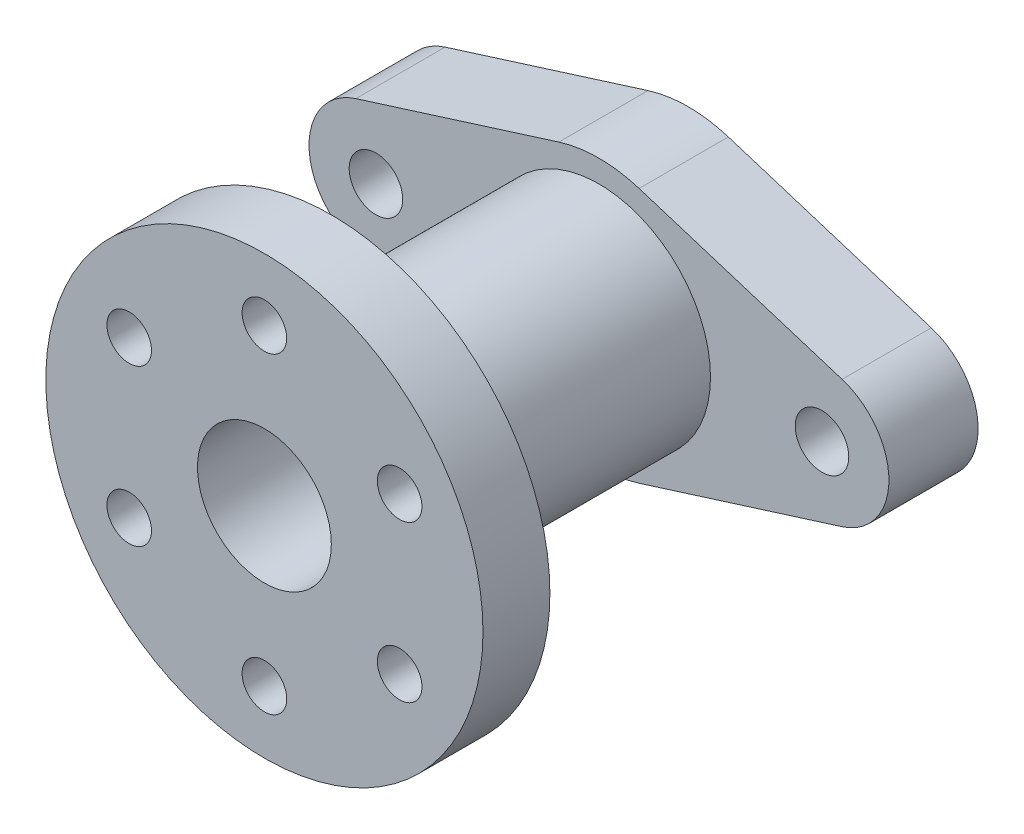
ISO-10303-21;
HEADER;
FILE_DESCRIPTION(('STEP AP214'),'2;1');
FILE_NAME('part.step','',(''),(''),'','','');
FILE_SCHEMA(('AUTOMOTIVE_DESIGN { 1 0 10303 214 1 1 1 1 }'));
ENDSEC;
DATA;
#1=APPLICATION_CONTEXT('core data for automotive mechanical design processes');
#2=APPLICATION_PROTOCOL_DEFINITION('international standard','automotive_design',2000,#1);
#3=PRODUCT_CONTEXT('',#1,'mechanical');
#4=PRODUCT('Part','Part','',(#3));
#5=PRODUCT_RELATED_PRODUCT_CATEGORY('part','',(#4));
#6=PRODUCT_DEFINITION_FORMATION('','',#4);
#7=PRODUCT_DEFINITION_CONTEXT('part definition',#1,'design');
#8=PRODUCT_DEFINITION('design','',#6,#7);
#9=PRODUCT_DEFINITION_SHAPE('','',#8);
#10=(LENGTH_UNIT() NAMED_UNIT(*) SI_UNIT(.MILLI.,.METRE.));
#11=(NAMED_UNIT(*) PLANE_ANGLE_UNIT() SI_UNIT($,.RADIAN.));
#12=(NAMED_UNIT(*) SI_UNIT($,.STERADIAN.) SOLID_ANGLE_UNIT());
#13=UNCERTAINTY_MEASURE_WITH_UNIT(LENGTH_MEASURE(1.E-05),#10,'distance_accuracy_value','');
#14=(GEOMETRIC_REPRESENTATION_CONTEXT(3) GLOBAL_UNCERTAINTY_ASSIGNED_CONTEXT((#13)) GLOBAL_UNIT_ASSIGNED_CONTEXT((#10,
#11,#12)) REPRESENTATION_CONTEXT('',''));
#15=CARTESIAN_POINT('',(0.,0.,0.));
#16=DIRECTION('',(0.,0.,1.));
#17=DIRECTION('',(1.,0.,0.));
#18=AXIS2_PLACEMENT_3D('',#15,#16,#17);
#19=CARTESIAN_POINT('',(0.,0.,20.));
#20=DIRECTION('',(0.,0.,-1.));
#21=DIRECTION('',(-1.,0.,0.));
#22=AXIS2_PLACEMENT_3D('',#19,#20,#21);
#23=CYLINDRICAL_SURFACE('',#22,15.);
#24=CARTESIAN_POINT('',(0.,0.,0.));
#25=DIRECTION('',(0.,0.,1.));
#26=DIRECTION('',(1.,0.,0.));
#27=AXIS2_PLACEMENT_3D('',#24,#25,#26);
#28=CIRCLE('',#27,15.);
#29=CARTESIAN_POINT('',(-4.5,14.3090880212542,0.));
#30=VERTEX_POINT('',#29);
#31=CARTESIAN_POINT('',(-4.5,-14.3090880212542,0.));
#32=VERTEX_POINT('',#31);
#33=EDGE_CURVE('E140',#30,#32,#28,.T.);
#34=ORIENTED_EDGE('',*,*,#33,.T.);
#35=DIRECTION('',(0.,0.,-1.));
#36=VECTOR('',#35,1.);
#37=CARTESIAN_POINT('',(-4.5,-14.3090880212542,20.));
#38=LINE('',#37,#36);
#39=CARTESIAN_POINT('',(-4.5,-14.3090880212542,20.));
#40=VERTEX_POINT('',#39);
#41=EDGE_CURVE('E45',#40,#32,#38,.T.);
#42=ORIENTED_EDGE('',*,*,#41,.F.);
#43=CARTESIAN_POINT('',(0.,0.,20.));
#44=DIRECTION('',(0.,0.,1.));
#45=DIRECTION('',(1.,0.,0.));
#46=AXIS2_PLACEMENT_3D('',#43,#44,#45);
#47=CIRCLE('',#46,15.);
#48=CARTESIAN_POINT('',(-4.5,14.3090880212542,20.));
#49=VERTEX_POINT('',#48);
#50=EDGE_CURVE('E155',#49,#40,#47,.T.);
#51=ORIENTED_EDGE('',*,*,#50,.F.);
#52=DIRECTION('',(0.,0.,-1.));
#53=VECTOR('',#52,1.);
#54=CARTESIAN_POINT('',(-4.5,14.3090880212542,20.));
#55=LINE('',#54,#53);
#56=EDGE_CURVE('E131',#49,#30,#55,.T.);
#57=ORIENTED_EDGE('',*,*,#56,.T.);
#58=EDGE_LOOP('',(#34,#42,#51,#57));
#59=FACE_BOUND('',#58,.T.);
#60=ADVANCED_FACE('F39',(#59),#23,.T.);
#61=CARTESIAN_POINT('',(-4.5,-14.3090880212542,20.));
#62=DIRECTION('',(0.3,0.953939201416946,0.));
#63=DIRECTION('',(-0.953939201416946,0.3,0.));
#64=AXIS2_PLACEMENT_3D('',#61,#62,#63);
#65=PLANE('',#64);
#66=DIRECTION('',(0.953939201416946,-0.3,0.));
#67=VECTOR('',#66,1.);
#68=CARTESIAN_POINT('',(-4.5,-14.3090880212542,0.));
#69=LINE('',#68,#67);
#70=CARTESIAN_POINT('',(41.,-28.6181760425084,0.));
#71=VERTEX_POINT('',#70);
#72=EDGE_CURVE('E138',#32,#71,#69,.T.);
#73=ORIENTED_EDGE('',*,*,#72,.T.);
#74=DIRECTION('',(0.,0.,-1.));
#75=VECTOR('',#74,1.);
#76=CARTESIAN_POINT('',(41.,-28.6181760425084,20.));
#77=LINE('',#76,#75);
#78=CARTESIAN_POINT('',(41.,-28.6181760425084,20.));
#79=VERTEX_POINT('',#78);
#80=EDGE_CURVE('E161',#79,#71,#77,.T.);
#81=ORIENTED_EDGE('',*,*,#80,.F.);
#82=DIRECTION('',(0.953939201416946,-0.3,0.));
#83=VECTOR('',#82,1.);
#84=CARTESIAN_POINT('',(-4.5,-14.3090880212542,20.));
#85=LINE('',#84,#83);
#86=EDGE_CURVE('E99',#40,#79,#85,.T.);
#87=ORIENTED_EDGE('',*,*,#86,.F.);
#88=ORIENTED_EDGE('',*,*,#41,.T.);
#89=EDGE_LOOP('',(#73,#81,#87,#88));
#90=FACE_BOUND('',#89,.T.);
#91=ADVANCED_FACE('F170',(#90),#65,.F.);
#92=CARTESIAN_POINT('',(50.,0.,20.));
#93=DIRECTION('',(0.,0.,-1.));
#94=DIRECTION('',(-1.,0.,0.));
#95=AXIS2_PLACEMENT_3D('',#92,#93,#94);
#96=CYLINDRICAL_SURFACE('',#95,30.);
#97=CARTESIAN_POINT('',(50.,0.,0.));
#98=DIRECTION('',(0.,0.,1.));
#99=DIRECTION('',(1.,0.,0.));
#100=AXIS2_PLACEMENT_3D('',#97,#98,#99);
#101=CIRCLE('',#100,30.);
#102=CARTESIAN_POINT('',(59.,-28.6181760425084,0.));
#103=VERTEX_POINT('',#102);
#104=EDGE_CURVE('E141',#71,#103,#101,.T.);
#105=ORIENTED_EDGE('',*,*,#104,.T.);
#106=DIRECTION('',(0.,0.,-1.));
#107=VECTOR('',#106,1.);
#108=CARTESIAN_POINT('',(59.,-28.6181760425084,20.));
#109=LINE('',#108,#107);
#110=CARTESIAN_POINT('',(59.,-28.6181760425084,20.));
#111=VERTEX_POINT('',#110);
#112=EDGE_CURVE('E157',#111,#103,#109,.T.);
#113=ORIENTED_EDGE('',*,*,#112,.F.);
#114=CARTESIAN_POINT('',(50.,0.,20.));
#115=DIRECTION('',(0.,0.,1.));
#116=DIRECTION('',(1.,0.,0.));
#117=AXIS2_PLACEMENT_3D('',#114,#115,#116);
#118=CIRCLE('',#117,30.);
#119=EDGE_CURVE('E185',#79,#111,#118,.T.);
#120=ORIENTED_EDGE('',*,*,#119,.F.);
#121=ORIENTED_EDGE('',*,*,#80,.T.);
#122=EDGE_LOOP('',(#105,#113,#120,#121));
#123=FACE_BOUND('',#122,.T.);
#124=ADVANCED_FACE('F177',(#123),#96,.T.);
#125=CARTESIAN_POINT('',(59.,-28.6181760425084,20.));
#126=DIRECTION('',(-0.3,0.953939201416946,0.));
#127=DIRECTION('',(-0.953939201416946,-0.3,0.));
#128=AXIS2_PLACEMENT_3D('',#125,#126,#127);
#129=PLANE('',#128);
#130=DIRECTION('',(0.953939201416946,0.3,0.));
#131=VECTOR('',#130,1.);
#132=CARTESIAN_POINT('',(59.,-28.6181760425084,0.));
#133=LINE('',#132,#131);
#134=CARTESIAN_POINT('',(104.5,-14.3090880212542,0.));
#135=VERTEX_POINT('',#134);
#136=EDGE_CURVE('E144',#103,#135,#133,.T.);
#137=ORIENTED_EDGE('',*,*,#136,.T.);
#138=DIRECTION('',(0.,0.,-1.));
#139=VECTOR('',#138,1.);
#140=CARTESIAN_POINT('',(104.5,-14.3090880212542,20.));
#141=LINE('',#140,#139);
#142=CARTESIAN_POINT('',(104.5,-14.3090880212542,20.));
#143=VERTEX_POINT('',#142);
#144=EDGE_CURVE('E156',#143,#135,#141,.T.);
#145=ORIENTED_EDGE('',*,*,#144,.F.);
#146=DIRECTION('',(0.953939201416946,0.3,0.));
#147=VECTOR('',#146,1.);
#148=CARTESIAN_POINT('',(59.,-28.6181760425084,20.));
#149=LINE('',#148,#147);
#150=EDGE_CURVE('E182',#111,#143,#149,.T.);
#151=ORIENTED_EDGE('',*,*,#150,.F.);
#152=ORIENTED_EDGE('',*,*,#112,.T.);
#153=EDGE_LOOP('',(#137,#145,#151,#152));
#154=FACE_BOUND('',#153,.T.);
#155=ADVANCED_FACE('F176',(#154),#129,.F.);
#156=CARTESIAN_POINT('',(100.,0.,20.));
#157=DIRECTION('',(0.,0.,-1.));
#158=DIRECTION('',(-1.,0.,0.));
#159=AXIS2_PLACEMENT_3D('',#156,#157,#158);
#160=CYLINDRICAL_SURFACE('',#159,15.);
#161=CARTESIAN_POINT('',(100.,0.,0.));
#162=DIRECTION('',(0.,0.,1.));
#163=DIRECTION('',(1.,0.,0.));
#164=AXIS2_PLACEMENT_3D('',#161,#162,#163);
#165=CIRCLE('',#164,15.);
#166=CARTESIAN_POINT('',(104.5,14.3090880212542,0.));
#167=VERTEX_POINT('',#166);
#168=EDGE_CURVE('E150',#135,#167,#165,.T.);
#169=ORIENTED_EDGE('',*,*,#168,.T.);
#170=DIRECTION('',(0.,0.,-1.));
#171=VECTOR('',#170,1.);
#172=CARTESIAN_POINT('',(104.5,14.3090880212542,20.));
#173=LINE('',#172,#171);
#174=CARTESIAN_POINT('',(104.5,14.3090880212542,20.));
#175=VERTEX_POINT('',#174);
#176=EDGE_CURVE('E126',#175,#167,#173,.T.);
#177=ORIENTED_EDGE('',*,*,#176,.F.);
#178=CARTESIAN_POINT('',(100.,0.,20.));
#179=DIRECTION('',(0.,0.,1.));
#180=DIRECTION('',(1.,0.,0.));
#181=AXIS2_PLACEMENT_3D('',#178,#179,#180);
#182=CIRCLE('',#181,15.);
#183=EDGE_CURVE('E119',#143,#175,#182,.T.);
#184=ORIENTED_EDGE('',*,*,#183,.F.);
#185=ORIENTED_EDGE('',*,*,#144,.T.);
#186=EDGE_LOOP('',(#169,#177,#184,#185));
#187=FACE_BOUND('',#186,.T.);
#188=ADVANCED_FACE('F293',(#187),#160,.T.);
#189=CARTESIAN_POINT('',(59.,28.6181760425084,20.));
#190=DIRECTION('',(-0.3,-0.953939201416946,0.));
#191=DIRECTION('',(0.953939201416946,-0.3,0.));
#192=AXIS2_PLACEMENT_3D('',#189,#190,#191);
#193=PLANE('',#192);
#194=DIRECTION('',(-0.953939201416946,0.3,0.));
#195=VECTOR('',#194,1.);
#196=CARTESIAN_POINT('',(59.,28.6181760425084,0.));
#197=LINE('',#196,#195);
#198=CARTESIAN_POINT('',(59.,28.6181760425084,0.));
#199=VERTEX_POINT('',#198);
#200=EDGE_CURVE('E130',#167,#199,#197,.T.);
#201=ORIENTED_EDGE('',*,*,#200,.T.);
#202=DIRECTION('',(0.,0.,-1.));
#203=VECTOR('',#202,1.);
#204=CARTESIAN_POINT('',(59.,28.6181760425084,20.));
#205=LINE('',#204,#203);
#206=CARTESIAN_POINT('',(59.,28.6181760425084,20.));
#207=VERTEX_POINT('',#206);
#208=EDGE_CURVE('E121',#207,#199,#205,.T.);
#209=ORIENTED_EDGE('',*,*,#208,.F.);
#210=DIRECTION('',(-0.953939201416946,0.3,0.));
#211=VECTOR('',#210,1.);
#212=CARTESIAN_POINT('',(59.,28.6181760425084,20.));
#213=LINE('',#212,#211);
#214=EDGE_CURVE('E114',#175,#207,#213,.T.);
#215=ORIENTED_EDGE('',*,*,#214,.F.);
#216=ORIENTED_EDGE('',*,*,#176,.T.);
#217=EDGE_LOOP('',(#201,#209,#215,#216));
#218=FACE_BOUND('',#217,.T.);
#219=ADVANCED_FACE('F123',(#218),#193,.F.);
#220=CARTESIAN_POINT('',(50.,0.,20.));
#221=DIRECTION('',(0.,0.,-1.));
#222=DIRECTION('',(-1.,0.,0.));
#223=AXIS2_PLACEMENT_3D('',#220,#221,#222);
#224=CYLINDRICAL_SURFACE('',#223,30.);
#225=CARTESIAN_POINT('',(50.,0.,0.));
#226=DIRECTION('',(0.,0.,1.));
#227=DIRECTION('',(1.,0.,0.));
#228=AXIS2_PLACEMENT_3D('',#225,#226,#227);
#229=CIRCLE('',#228,30.);
#230=CARTESIAN_POINT('',(41.,28.6181760425084,0.));
#231=VERTEX_POINT('',#230);
#232=EDGE_CURVE('E83',#199,#231,#229,.T.);
#233=ORIENTED_EDGE('',*,*,#232,.T.);
#234=DIRECTION('',(0.,0.,-1.));
#235=VECTOR('',#234,1.);
#236=CARTESIAN_POINT('',(41.,28.6181760425084,20.));
#237=LINE('',#236,#235);
#238=CARTESIAN_POINT('',(41.,28.6181760425084,20.));
#239=VERTEX_POINT('',#238);
#240=EDGE_CURVE('E129',#239,#231,#237,.T.);
#241=ORIENTED_EDGE('',*,*,#240,.F.);
#242=CARTESIAN_POINT('',(50.,0.,20.));
#243=DIRECTION('',(0.,0.,1.));
#244=DIRECTION('',(1.,0.,0.));
#245=AXIS2_PLACEMENT_3D('',#242,#243,#244);
#246=CIRCLE('',#245,30.);
#247=EDGE_CURVE('E120',#207,#239,#246,.T.);
#248=ORIENTED_EDGE('',*,*,#247,.F.);
#249=ORIENTED_EDGE('',*,*,#208,.T.);
#250=EDGE_LOOP('',(#233,#241,#248,#249));
#251=FACE_BOUND('',#250,.T.);
#252=ADVANCED_FACE('F133',(#251),#224,.T.);
#253=CARTESIAN_POINT('',(-4.5,14.3090880212542,20.));
#254=DIRECTION('',(0.3,-0.953939201416946,0.));
#255=DIRECTION('',(0.953939201416946,0.3,0.));
#256=AXIS2_PLACEMENT_3D('',#253,#254,#255);
#257=PLANE('',#256);
#258=DIRECTION('',(-0.953939201416946,-0.3,0.));
#259=VECTOR('',#258,1.);
#260=CARTESIAN_POINT('',(-4.5,14.3090880212542,0.));
#261=LINE('',#260,#259);
#262=EDGE_CURVE('E93',#231,#30,#261,.T.);
#263=ORIENTED_EDGE('',*,*,#262,.T.);
#264=ORIENTED_EDGE('',*,*,#56,.F.);
#265=DIRECTION('',(-0.953939201416946,-0.3,0.));
#266=VECTOR('',#265,1.);
#267=CARTESIAN_POINT('',(-4.5,14.3090880212542,20.));
#268=LINE('',#267,#266);
#269=EDGE_CURVE('E57',#239,#49,#268,.T.);
#270=ORIENTED_EDGE('',*,*,#269,.F.);
#271=ORIENTED_EDGE('',*,*,#240,.T.);
#272=EDGE_LOOP('',(#263,#264,#270,#271));
#273=FACE_BOUND('',#272,.T.);
#274=ADVANCED_FACE('F265',(#273),#257,.F.);
#275=CARTESIAN_POINT('',(0.,0.,20.));
#276=DIRECTION('',(0.,0.,1.));
#277=DIRECTION('',(1.,0.,0.));
#278=AXIS2_PLACEMENT_3D('',#275,#276,#277);
#279=PLANE('',#278);
#280=CARTESIAN_POINT('',(0.,0.,20.));
#281=DIRECTION('',(0.,0.,1.));
#282=DIRECTION('',(1.,0.,0.));
#283=AXIS2_PLACEMENT_3D('',#280,#281,#282);
#284=CIRCLE('',#283,6.);
#285=CARTESIAN_POINT('',(6.,0.,20.));
#286=VERTEX_POINT('',#285);
#287=EDGE_CURVE('E242',#286,#286,#284,.T.);
#288=ORIENTED_EDGE('',*,*,#287,.F.);
#289=EDGE_LOOP('',(#288));
#290=FACE_BOUND('',#289,.T.);
#291=CARTESIAN_POINT('',(100.,0.,20.));
#292=DIRECTION('',(0.,0.,1.));
#293=DIRECTION('',(1.,0.,0.));
#294=AXIS2_PLACEMENT_3D('',#291,#292,#293);
#295=CIRCLE('',#294,6.);
#296=CARTESIAN_POINT('',(106.,0.,20.));
#297=VERTEX_POINT('',#296);
#298=EDGE_CURVE('E239',#297,#297,#295,.T.);
#299=ORIENTED_EDGE('',*,*,#298,.F.);
#300=EDGE_LOOP('',(#299));
#301=FACE_BOUND('',#300,.T.);
#302=CARTESIAN_POINT('',(50.,0.,20.));
#303=DIRECTION('',(0.,0.,1.));
#304=DIRECTION('',(1.,0.,0.));
#305=AXIS2_PLACEMENT_3D('',#302,#303,#304);
#306=CIRCLE('',#305,25.);
#307=CARTESIAN_POINT('',(75.,0.,20.));
#308=VERTEX_POINT('',#307);
#309=EDGE_CURVE('E11',#308,#308,#306,.T.);
#310=ORIENTED_EDGE('',*,*,#309,.F.);
#311=EDGE_LOOP('',(#310));
#312=FACE_BOUND('',#311,.T.);
#313=ORIENTED_EDGE('',*,*,#50,.T.);
#314=ORIENTED_EDGE('',*,*,#86,.T.);
#315=ORIENTED_EDGE('',*,*,#119,.T.);
#316=ORIENTED_EDGE('',*,*,#150,.T.);
#317=ORIENTED_EDGE('',*,*,#183,.T.);
#318=ORIENTED_EDGE('',*,*,#214,.T.);
#319=ORIENTED_EDGE('',*,*,#247,.T.);
#320=ORIENTED_EDGE('',*,*,#269,.T.);
#321=EDGE_LOOP('',(#313,#314,#315,#316,#317,#318,#319,#320));
#322=FACE_BOUND('',#321,.T.);
#323=ADVANCED_FACE('F113',(#290,#301,#312,#322),#279,.T.);
#324=CARTESIAN_POINT('',(0.,0.,0.));
#325=DIRECTION('',(0.,0.,1.));
#326=DIRECTION('',(1.,0.,0.));
#327=AXIS2_PLACEMENT_3D('',#324,#325,#326);
#328=PLANE('',#327);
#329=CARTESIAN_POINT('',(50.,0.,0.));
#330=DIRECTION('',(0.,0.,1.));
#331=DIRECTION('',(1.,0.,0.));
#332=AXIS2_PLACEMENT_3D('',#329,#330,#331);
#333=CIRCLE('',#332,15.);
#334=CARTESIAN_POINT('',(65.,0.,0.));
#335=VERTEX_POINT('',#334);
#336=EDGE_CURVE('E199',#335,#335,#333,.T.);
#337=ORIENTED_EDGE('',*,*,#336,.T.);
#338=EDGE_LOOP('',(#337));
#339=FACE_BOUND('',#338,.T.);
#340=ORIENTED_EDGE('',*,*,#33,.F.);
#341=ORIENTED_EDGE('',*,*,#262,.F.);
#342=ORIENTED_EDGE('',*,*,#232,.F.);
#343=ORIENTED_EDGE('',*,*,#200,.F.);
#344=ORIENTED_EDGE('',*,*,#168,.F.);
#345=ORIENTED_EDGE('',*,*,#136,.F.);
#346=ORIENTED_EDGE('',*,*,#104,.F.);
#347=ORIENTED_EDGE('',*,*,#72,.F.);
#348=EDGE_LOOP('',(#340,#341,#342,#343,#344,#345,#346,#347));
#349=FACE_BOUND('',#348,.T.);
#350=ADVANCED_FACE('F175',(#339,#349),#328,.F.);
#351=CARTESIAN_POINT('',(50.,0.,80.));
#352=DIRECTION('',(0.,0.,-1.));
#353=DIRECTION('',(-1.,0.,0.));
#354=AXIS2_PLACEMENT_3D('',#351,#352,#353);
#355=CYLINDRICAL_SURFACE('',#354,25.);
#356=CARTESIAN_POINT('',(50.,0.,80.));
#357=DIRECTION('',(0.,0.,1.));
#358=DIRECTION('',(1.,0.,0.));
#359=AXIS2_PLACEMENT_3D('',#356,#357,#358);
#360=CIRCLE('',#359,25.);
#361=CARTESIAN_POINT('',(75.,0.,80.));
#362=VERTEX_POINT('',#361);
#363=EDGE_CURVE('E143',#362,#362,#360,.T.);
#364=ORIENTED_EDGE('',*,*,#363,.F.);
#365=EDGE_LOOP('',(#364));
#366=FACE_BOUND('',#365,.T.);
#367=ORIENTED_EDGE('',*,*,#309,.T.);
#368=EDGE_LOOP('',(#367));
#369=FACE_BOUND('',#368,.T.);
#370=ADVANCED_FACE('F268',(#366,#369),#355,.T.);
#371=CARTESIAN_POINT('',(50.,0.,95.));
#372=DIRECTION('',(0.,0.,-1.));
#373=DIRECTION('',(-1.,0.,0.));
#374=AXIS2_PLACEMENT_3D('',#371,#372,#373);
#375=CYLINDRICAL_SURFACE('',#374,49.);
#376=CARTESIAN_POINT('',(50.,0.,95.));
#377=DIRECTION('',(0.,0.,1.));
#378=DIRECTION('',(1.,0.,0.));
#379=AXIS2_PLACEMENT_3D('',#376,#377,#378);
#380=CIRCLE('',#379,49.);
#381=CARTESIAN_POINT('',(99.,0.,95.));
#382=VERTEX_POINT('',#381);
#383=EDGE_CURVE('E187',#382,#382,#380,.T.);
#384=ORIENTED_EDGE('',*,*,#383,.F.);
#385=EDGE_LOOP('',(#384));
#386=FACE_BOUND('',#385,.T.);
#387=CARTESIAN_POINT('',(50.,0.,80.));
#388=DIRECTION('',(0.,0.,1.));
#389=DIRECTION('',(1.,0.,0.));
#390=AXIS2_PLACEMENT_3D('',#387,#388,#389);
#391=CIRCLE('',#390,49.);
#392=CARTESIAN_POINT('',(99.,0.,80.));
#393=VERTEX_POINT('',#392);
#394=EDGE_CURVE('E192',#393,#393,#391,.T.);
#395=ORIENTED_EDGE('',*,*,#394,.T.);
#396=EDGE_LOOP('',(#395));
#397=FACE_BOUND('',#396,.T.);
#398=ADVANCED_FACE('F269',(#386,#397),#375,.T.);
#399=CARTESIAN_POINT('',(50.,0.,95.));
#400=DIRECTION('',(0.,0.,1.));
#401=DIRECTION('',(1.,0.,0.));
#402=AXIS2_PLACEMENT_3D('',#399,#400,#401);
#403=PLANE('',#402);
#404=CARTESIAN_POINT('',(19.6891108675449,17.5000000000003,95.));
#405=DIRECTION('',(0.,0.,1.));
#406=DIRECTION('',(0.50000000000001,0.866025403784433,0.));
#407=AXIS2_PLACEMENT_3D('',#404,#405,#406);
#408=CIRCLE('',#407,5.00000000000001);
#409=CARTESIAN_POINT('',(22.1891108675449,21.8301270189225,95.));
#410=VERTEX_POINT('',#409);
#411=EDGE_CURVE('E214',#410,#410,#408,.T.);
#412=ORIENTED_EDGE('',*,*,#411,.F.);
#413=EDGE_LOOP('',(#412));
#414=FACE_BOUND('',#413,.T.);
#415=CARTESIAN_POINT('',(19.6891108675445,-17.4999999999997,95.));
#416=DIRECTION('',(0.,0.,1.));
#417=DIRECTION('',(-0.499999999999992,0.866025403784443,0.));
#418=AXIS2_PLACEMENT_3D('',#415,#416,#417);
#419=CIRCLE('',#418,5.00000000000001);
#420=CARTESIAN_POINT('',(17.1891108675445,-13.1698729810775,95.));
#421=VERTEX_POINT('',#420);
#422=EDGE_CURVE('E225',#421,#421,#419,.T.);
#423=ORIENTED_EDGE('',*,*,#422,.F.);
#424=EDGE_LOOP('',(#423));
#425=FACE_BOUND('',#424,.T.);
#426=CARTESIAN_POINT('',(50.,-35.,95.));
#427=DIRECTION('',(0.,0.,1.));
#428=DIRECTION('',(-1.,0.,0.));
#429=AXIS2_PLACEMENT_3D('',#426,#427,#428);
#430=CIRCLE('',#429,5.00000000000001);
#431=CARTESIAN_POINT('',(45.,-35.,95.));
#432=VERTEX_POINT('',#431);
#433=EDGE_CURVE('E226',#432,#432,#430,.T.);
#434=ORIENTED_EDGE('',*,*,#433,.F.);
#435=EDGE_LOOP('',(#434));
#436=FACE_BOUND('',#435,.T.);
#437=CARTESIAN_POINT('',(80.3108891324553,-17.5000000000001,95.));
#438=DIRECTION('',(0.,0.,1.));
#439=DIRECTION('',(-0.500000000000004,-0.866025403784436,0.));
#440=AXIS2_PLACEMENT_3D('',#437,#438,#439);
#441=CIRCLE('',#440,5.00000000000001);
#442=CARTESIAN_POINT('',(77.8108891324552,-21.8301270189223,95.));
#443=VERTEX_POINT('',#442);
#444=EDGE_CURVE('E231',#443,#443,#441,.T.);
#445=ORIENTED_EDGE('',*,*,#444,.F.);
#446=EDGE_LOOP('',(#445));
#447=FACE_BOUND('',#446,.T.);
#448=CARTESIAN_POINT('',(80.3108891324554,17.4999999999999,95.));
#449=DIRECTION('',(0.,0.,1.));
#450=DIRECTION('',(0.499999999999998,-0.86602540378444,0.));
#451=AXIS2_PLACEMENT_3D('',#448,#449,#450);
#452=CIRCLE('',#451,5.00000000000001);
#453=CARTESIAN_POINT('',(82.8108891324554,13.1698729810777,95.));
#454=VERTEX_POINT('',#453);
#455=EDGE_CURVE('E207',#454,#454,#452,.T.);
#456=ORIENTED_EDGE('',*,*,#455,.F.);
#457=EDGE_LOOP('',(#456));
#458=FACE_BOUND('',#457,.T.);
#459=CARTESIAN_POINT('',(50.,0.,95.));
#460=DIRECTION('',(0.,0.,1.));
#461=DIRECTION('',(1.,0.,0.));
#462=AXIS2_PLACEMENT_3D('',#459,#460,#461);
#463=CIRCLE('',#462,15.);
#464=CARTESIAN_POINT('',(65.,0.,95.));
#465=VERTEX_POINT('',#464);
#466=EDGE_CURVE('E201',#465,#465,#463,.T.);
#467=ORIENTED_EDGE('',*,*,#466,.F.);
#468=EDGE_LOOP('',(#467));
#469=FACE_BOUND('',#468,.T.);
#470=CARTESIAN_POINT('',(50.,35.,95.));
#471=DIRECTION('',(0.,0.,1.));
#472=DIRECTION('',(1.,0.,0.));
#473=AXIS2_PLACEMENT_3D('',#470,#471,#472);
#474=CIRCLE('',#473,5.00000000000001);
#475=CARTESIAN_POINT('',(55.,35.,95.));
#476=VERTEX_POINT('',#475);
#477=EDGE_CURVE('E197',#476,#476,#474,.T.);
#478=ORIENTED_EDGE('',*,*,#477,.F.);
#479=EDGE_LOOP('',(#478));
#480=FACE_BOUND('',#479,.T.);
#481=ORIENTED_EDGE('',*,*,#383,.T.);
#482=EDGE_LOOP('',(#481));
#483=FACE_BOUND('',#482,.T.);
#484=ADVANCED_FACE('F280',(#414,#425,#436,#447,#458,#469,#480,#483),#403,.T.);
#485=CARTESIAN_POINT('',(50.,0.,80.));
#486=DIRECTION('',(0.,0.,1.));
#487=DIRECTION('',(1.,0.,0.));
#488=AXIS2_PLACEMENT_3D('',#485,#486,#487);
#489=PLANE('',#488);
#490=CARTESIAN_POINT('',(19.6891108675449,17.5000000000003,80.));
#491=DIRECTION('',(0.,0.,1.));
#492=DIRECTION('',(0.50000000000001,0.866025403784433,0.));
#493=AXIS2_PLACEMENT_3D('',#490,#491,#492);
#494=CIRCLE('',#493,5.00000000000001);
#495=CARTESIAN_POINT('',(22.1891108675449,21.8301270189225,80.));
#496=VERTEX_POINT('',#495);
#497=EDGE_CURVE('E217',#496,#496,#494,.T.);
#498=ORIENTED_EDGE('',*,*,#497,.T.);
#499=EDGE_LOOP('',(#498));
#500=FACE_BOUND('',#499,.T.);
#501=CARTESIAN_POINT('',(19.6891108675445,-17.4999999999997,80.));
#502=DIRECTION('',(0.,0.,1.));
#503=DIRECTION('',(-0.499999999999992,0.866025403784443,0.));
#504=AXIS2_PLACEMENT_3D('',#501,#502,#503);
#505=CIRCLE('',#504,5.00000000000001);
#506=CARTESIAN_POINT('',(17.1891108675445,-13.1698729810775,80.));
#507=VERTEX_POINT('',#506);
#508=EDGE_CURVE('E223',#507,#507,#505,.T.);
#509=ORIENTED_EDGE('',*,*,#508,.T.);
#510=EDGE_LOOP('',(#509));
#511=FACE_BOUND('',#510,.T.);
#512=CARTESIAN_POINT('',(50.,-35.,80.));
#513=DIRECTION('',(0.,0.,1.));
#514=DIRECTION('',(-1.,0.,0.));
#515=AXIS2_PLACEMENT_3D('',#512,#513,#514);
#516=CIRCLE('',#515,5.00000000000001);
#517=CARTESIAN_POINT('',(45.,-35.,80.));
#518=VERTEX_POINT('',#517);
#519=EDGE_CURVE('E232',#518,#518,#516,.T.);
#520=ORIENTED_EDGE('',*,*,#519,.T.);
#521=EDGE_LOOP('',(#520));
#522=FACE_BOUND('',#521,.T.);
#523=CARTESIAN_POINT('',(80.3108891324553,-17.5000000000001,80.));
#524=DIRECTION('',(0.,0.,1.));
#525=DIRECTION('',(-0.500000000000004,-0.866025403784436,0.));
#526=AXIS2_PLACEMENT_3D('',#523,#524,#525);
#527=CIRCLE('',#526,5.00000000000001);
#528=CARTESIAN_POINT('',(77.8108891324552,-21.8301270189223,80.));
#529=VERTEX_POINT('',#528);
#530=EDGE_CURVE('E215',#529,#529,#527,.T.);
#531=ORIENTED_EDGE('',*,*,#530,.T.);
#532=EDGE_LOOP('',(#531));
#533=FACE_BOUND('',#532,.T.);
#534=CARTESIAN_POINT('',(80.3108891324554,17.4999999999999,80.));
#535=DIRECTION('',(0.,0.,1.));
#536=DIRECTION('',(0.499999999999998,-0.86602540378444,0.));
#537=AXIS2_PLACEMENT_3D('',#534,#535,#536);
#538=CIRCLE('',#537,5.00000000000001);
#539=CARTESIAN_POINT('',(82.8108891324554,13.1698729810777,80.));
#540=VERTEX_POINT('',#539);
#541=EDGE_CURVE('E206',#540,#540,#538,.T.);
#542=ORIENTED_EDGE('',*,*,#541,.T.);
#543=EDGE_LOOP('',(#542));
#544=FACE_BOUND('',#543,.T.);
#545=CARTESIAN_POINT('',(50.,35.,80.));
#546=DIRECTION('',(0.,0.,1.));
#547=DIRECTION('',(1.,0.,0.));
#548=AXIS2_PLACEMENT_3D('',#545,#546,#547);
#549=CIRCLE('',#548,5.00000000000001);
#550=CARTESIAN_POINT('',(55.,35.,80.));
#551=VERTEX_POINT('',#550);
#552=EDGE_CURVE('E191',#551,#551,#549,.T.);
#553=ORIENTED_EDGE('',*,*,#552,.T.);
#554=EDGE_LOOP('',(#553));
#555=FACE_BOUND('',#554,.T.);
#556=ORIENTED_EDGE('',*,*,#363,.T.);
#557=EDGE_LOOP('',(#556));
#558=FACE_BOUND('',#557,.T.);
#559=ORIENTED_EDGE('',*,*,#394,.F.);
#560=EDGE_LOOP('',(#559));
#561=FACE_BOUND('',#560,.T.);
#562=ADVANCED_FACE('F371',(#500,#511,#522,#533,#544,#555,#558,#561),#489,.F.);
#563=CARTESIAN_POINT('',(50.,35.,80.));
#564=DIRECTION('',(0.,0.,1.));
#565=DIRECTION('',(1.,0.,0.));
#566=AXIS2_PLACEMENT_3D('',#563,#564,#565);
#567=CYLINDRICAL_SURFACE('',#566,5.00000000000001);
#568=ORIENTED_EDGE('',*,*,#552,.F.);
#569=EDGE_LOOP('',(#568));
#570=FACE_BOUND('',#569,.T.);
#571=ORIENTED_EDGE('',*,*,#477,.T.);
#572=EDGE_LOOP('',(#571));
#573=FACE_BOUND('',#572,.T.);
#574=ADVANCED_FACE('F379',(#570,#573),#567,.F.);
#575=CARTESIAN_POINT('',(50.,0.,0.));
#576=DIRECTION('',(0.,0.,1.));
#577=DIRECTION('',(1.,0.,0.));
#578=AXIS2_PLACEMENT_3D('',#575,#576,#577);
#579=CYLINDRICAL_SURFACE('',#578,15.);
#580=ORIENTED_EDGE('',*,*,#336,.F.);
#581=EDGE_LOOP('',(#580));
#582=FACE_BOUND('',#581,.T.);
#583=ORIENTED_EDGE('',*,*,#466,.T.);
#584=EDGE_LOOP('',(#583));
#585=FACE_BOUND('',#584,.T.);
#586=ADVANCED_FACE('F386',(#582,#585),#579,.F.);
#587=CARTESIAN_POINT('',(80.3108891324554,17.4999999999999,80.));
#588=DIRECTION('',(0.,0.,1.));
#589=DIRECTION('',(1.,0.,0.));
#590=AXIS2_PLACEMENT_3D('',#587,#588,#589);
#591=CYLINDRICAL_SURFACE('',#590,5.00000000000001);
#592=ORIENTED_EDGE('',*,*,#541,.F.);
#593=EDGE_LOOP('',(#592));
#594=FACE_BOUND('',#593,.T.);
#595=ORIENTED_EDGE('',*,*,#455,.T.);
#596=EDGE_LOOP('',(#595));
#597=FACE_BOUND('',#596,.T.);
#598=ADVANCED_FACE('F399',(#594,#597),#591,.F.);
#599=CARTESIAN_POINT('',(80.3108891324553,-17.5000000000001,80.));
#600=DIRECTION('',(0.,0.,1.));
#601=DIRECTION('',(1.,0.,0.));
#602=AXIS2_PLACEMENT_3D('',#599,#600,#601);
#603=CYLINDRICAL_SURFACE('',#602,5.00000000000001);
#604=ORIENTED_EDGE('',*,*,#530,.F.);
#605=EDGE_LOOP('',(#604));
#606=FACE_BOUND('',#605,.T.);
#607=ORIENTED_EDGE('',*,*,#444,.T.);
#608=EDGE_LOOP('',(#607));
#609=FACE_BOUND('',#608,.T.);
#610=ADVANCED_FACE('F410',(#606,#609),#603,.F.);
#611=CARTESIAN_POINT('',(50.,-35.,80.));
#612=DIRECTION('',(0.,0.,1.));
#613=DIRECTION('',(1.,0.,0.));
#614=AXIS2_PLACEMENT_3D('',#611,#612,#613);
#615=CYLINDRICAL_SURFACE('',#614,5.00000000000001);
#616=ORIENTED_EDGE('',*,*,#519,.F.);
#617=EDGE_LOOP('',(#616));
#618=FACE_BOUND('',#617,.T.);
#619=ORIENTED_EDGE('',*,*,#433,.T.);
#620=EDGE_LOOP('',(#619));
#621=FACE_BOUND('',#620,.T.);
#622=ADVANCED_FACE('F418',(#618,#621),#615,.F.);
#623=CARTESIAN_POINT('',(19.6891108675445,-17.4999999999997,80.));
#624=DIRECTION('',(0.,0.,1.));
#625=DIRECTION('',(1.,0.,0.));
#626=AXIS2_PLACEMENT_3D('',#623,#624,#625);
#627=CYLINDRICAL_SURFACE('',#626,5.00000000000001);
#628=ORIENTED_EDGE('',*,*,#508,.F.);
#629=EDGE_LOOP('',(#628));
#630=FACE_BOUND('',#629,.T.);
#631=ORIENTED_EDGE('',*,*,#422,.T.);
#632=EDGE_LOOP('',(#631));
#633=FACE_BOUND('',#632,.T.);
#634=ADVANCED_FACE('F422',(#630,#633),#627,.F.);
#635=CARTESIAN_POINT('',(19.6891108675449,17.5000000000003,80.));
#636=DIRECTION('',(0.,0.,1.));
#637=DIRECTION('',(1.,0.,0.));
#638=AXIS2_PLACEMENT_3D('',#635,#636,#637);
#639=CYLINDRICAL_SURFACE('',#638,5.00000000000001);
#640=ORIENTED_EDGE('',*,*,#497,.F.);
#641=EDGE_LOOP('',(#640));
#642=FACE_BOUND('',#641,.T.);
#643=ORIENTED_EDGE('',*,*,#411,.T.);
#644=EDGE_LOOP('',(#643));
#645=FACE_BOUND('',#644,.T.);
#646=ADVANCED_FACE('F432',(#642,#645),#639,.F.);
#647=CARTESIAN_POINT('',(100.,0.,5.));
#648=DIRECTION('',(0.,0.,1.));
#649=DIRECTION('',(1.,0.,0.));
#650=AXIS2_PLACEMENT_3D('',#647,#648,#649);
#651=CYLINDRICAL_SURFACE('',#650,6.);
#652=CARTESIAN_POINT('',(100.,0.,5.));
#653=DIRECTION('',(0.,0.,1.));
#654=DIRECTION('',(1.,0.,0.));
#655=AXIS2_PLACEMENT_3D('',#652,#653,#654);
#656=CIRCLE('',#655,6.);
#657=CARTESIAN_POINT('',(106.,0.,5.));
#658=VERTEX_POINT('',#657);
#659=EDGE_CURVE('E245',#658,#658,#656,.T.);
#660=ORIENTED_EDGE('',*,*,#659,.F.);
#661=EDGE_LOOP('',(#660));
#662=FACE_BOUND('',#661,.T.);
#663=ORIENTED_EDGE('',*,*,#298,.T.);
#664=EDGE_LOOP('',(#663));
#665=FACE_BOUND('',#664,.T.);
#666=ADVANCED_FACE('F444',(#662,#665),#651,.F.);
#667=CARTESIAN_POINT('',(100.,0.,5.));
#668=DIRECTION('',(0.,0.,1.));
#669=DIRECTION('',(1.,0.,0.));
#670=AXIS2_PLACEMENT_3D('',#667,#668,#669);
#671=PLANE('',#670);
#672=ORIENTED_EDGE('',*,*,#659,.T.);
#673=EDGE_LOOP('',(#672));
#674=FACE_BOUND('',#673,.T.);
#675=ADVANCED_FACE('F258',(#674),#671,.T.);
#676=CARTESIAN_POINT('',(0.,0.,5.));
#677=DIRECTION('',(0.,0.,1.));
#678=DIRECTION('',(1.,0.,0.));
#679=AXIS2_PLACEMENT_3D('',#676,#677,#678);
#680=CYLINDRICAL_SURFACE('',#679,6.);
#681=CARTESIAN_POINT('',(0.,0.,5.));
#682=DIRECTION('',(0.,0.,1.));
#683=DIRECTION('',(1.,0.,0.));
#684=AXIS2_PLACEMENT_3D('',#681,#682,#683);
#685=CIRCLE('',#684,6.);
#686=CARTESIAN_POINT('',(6.,0.,5.));
#687=VERTEX_POINT('',#686);
#688=EDGE_CURVE('E218',#687,#687,#685,.T.);
#689=ORIENTED_EDGE('',*,*,#688,.F.);
#690=EDGE_LOOP('',(#689));
#691=FACE_BOUND('',#690,.T.);
#692=ORIENTED_EDGE('',*,*,#287,.T.);
#693=EDGE_LOOP('',(#692));
#694=FACE_BOUND('',#693,.T.);
#695=ADVANCED_FACE('F251',(#691,#694),#680,.F.);
#696=CARTESIAN_POINT('',(0.,0.,5.));
#697=DIRECTION('',(0.,0.,1.));
#698=DIRECTION('',(1.,0.,0.));
#699=AXIS2_PLACEMENT_3D('',#696,#697,#698);
#700=PLANE('',#699);
#701=ORIENTED_EDGE('',*,*,#688,.T.);
#702=EDGE_LOOP('',(#701));
#703=FACE_BOUND('',#702,.T.);
#704=ADVANCED_FACE('F253',(#703),#700,.T.);
#705=CLOSED_SHELL('',(#60,#91,#124,#155,#188,#219,#252,#274,#323,#350,#370,#398,#484,#562,#574,
#586,#598,#610,#622,#634,#646,#666,#675,#695,#704));
#706=MANIFOLD_SOLID_BREP('B2',#705);
#707=ADVANCED_BREP_SHAPE_REPRESENTATION('',(#18,#706),#14);
#708=SHAPE_DEFINITION_REPRESENTATION(#9,#707);
ENDSEC;
END-ISO-10303-21;
